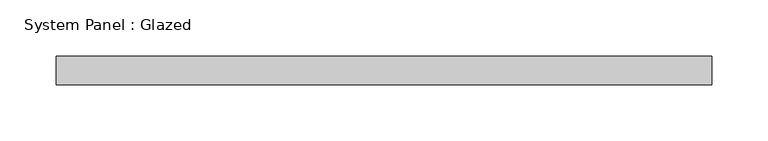
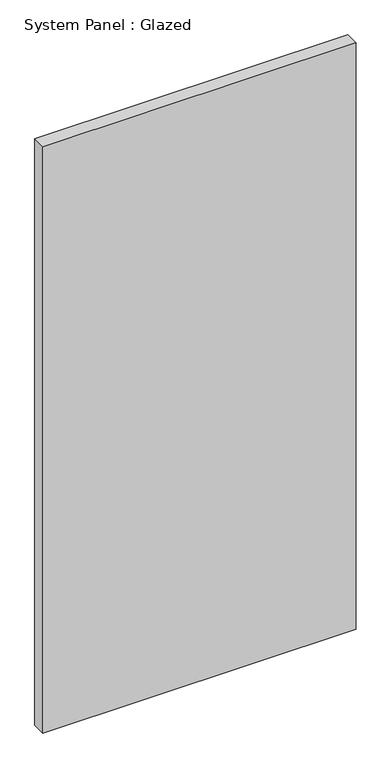
"""IFC4 building model written with IfcOpenShell, lengths in millimetres: plate geometry, System Panel : Glazed."""

from ifc_helpers import new_model, si_unit, origin, origin_with_axes, place, context, project, spatial, polyline, outline, extrude, source, transform, mapped, element, save


def system_panel_glazed_da164243(model_context):
    return source(origin(), model_context, "Body", "SweptSolid", [
        extrude(outline(polyline([(292.1, 19.05), (-292.1, 19.05), (-292.1, 44.45), (292.1, 44.45), (292.1, 19.05)])), origin_with_axes(), (0.0, 0.0, 1.0), 1155.7),
    ])


if __name__ == "__main__":
    model = new_model("IFC4")
    model_context = context("Model", 3, world=origin())
    ifc_project = project(units=[si_unit("LENGTHUNIT", "METRE", prefix="MILLI")], contexts=[model_context])
    site = spatial("IfcSite", under=ifc_project)
    building = spatial("IfcBuilding", under=site)
    placement = place(None, origin())
    system_panel_glazed_shape = system_panel_glazed_da164243(model_context)
    element("IfcPlate", 1, ObjectType="System Panel : Glazed", at=placement, inside=building, context=model_context, shape_type="MappedRepresentation", body=[
        mapped(system_panel_glazed_shape, transform((0.0, 0.0, 0.0), x_axis=(1.0, 0.0, 0.0), y_axis=(0.0, 1.0, 0.0), z_axis=(0.0, 0.0, 1.0))),
    ])
    save(model, "model.ifc")

# Revit data of these elements
# Type "System Panel : Glazed"
#   Construction Type Id = "GSP4R"
#   Analytic Construction = "1/8 in Pilkington single glazing"
#   Visual Light Transmittance = 0.9
#   Solar Heat Gain Coefficient = 0.86
#   Heat Transfer Coefficient (U) = 1.18115 BTU/(h·ft²·°F)
# Element 1 (IfcPlate, "System Panel : Glazed")
#   Materials on its faces: "Glass"
# Materials
#   "Glass": class "Glass", colour RGB 0 128 192, transparency 0.75, Description = "Soda Lime Glass", Cost = 0
